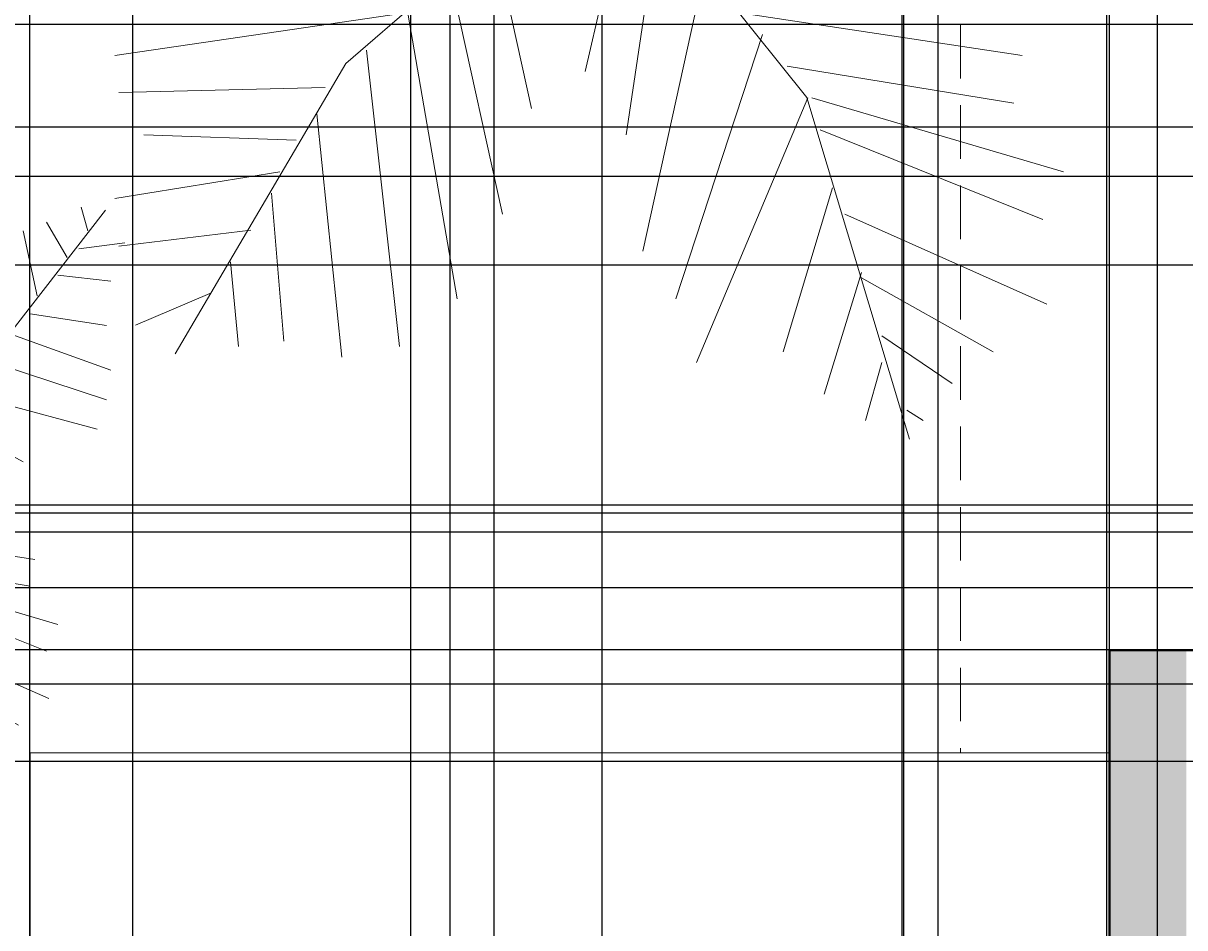
# Model space of a CAD drawing. Units: inches. Extents: x 818 to 1898, y 976 to 2364.
# Tile 11 of 96: x 1071 to 1207, y 1668 to 1773. Entities that reach past the tile are written whole.
import ezdxf

# ---------------------------------------------------------------- set-up
doc = ezdxf.new("R2010")
doc.units = ezdxf.units.IN
doc.header["$LTSCALE"] = 5
doc.header["$MEASUREMENT"] = 0
doc.linetypes.add('HIDDEN', pattern=[0.375, 0.25, -0.125])
for name, color, linetype, lineweight in [('A-ANNO-DIMS', 2, 'Continuous', 18), ('A-FLOR-OVHD', 8, 'HIDDEN', 13), ('A-WALL', 7, 'Continuous', 40), ('L-PAVE', 8, 'Continuous', 18), ('L-PLNT-BEDS', 94, 'Continuous', 18)]:
    doc.layers.add(name, color=color, linetype=linetype, lineweight=lineweight)
doc.layers.add('A-WALL-PATT', color=251, linetype='Continuous', lineweight=13, true_color=0x636466)
doc.layers.add('L-PLNT', color=116, linetype='Continuous', lineweight=13, true_color=0x136734)
doc.styles.get("Standard").update_dxf_attribs({"font": 'arial.ttf'})
doc.dimstyles.get("Standard").update_dxf_attribs({"dimtxt": 0.18, "dimasz": 0.18, "dimexe": 0.18, "dimexo": 0.0625, "dimgap": 0.09, "dimtad": 0, "dimtih": 1, "dimtoh": 1, "dimdec": 4, "dimzin": 0, "dimdsep": 46, "dimtxsty": 'Standard', "dimcen": 0.09, "dimadec": 0, "dimazin": 0, "dimtfac": 1, "dimtdec": 4, "dimtofl": 0, "dimtmove": 0, "dimatfit": 3, "dimfxl": 1, "dimtolj": 1, "dimtzin": 0, "dimarcsym": 0})

# ---------------------------------------------------------------- blocks, each defined once
blk = doc.blocks.new('PALM-BORDER')
for p, q in [((41.53, 39.05), (33.72, 81.45)), ((33.95, 78.95), (31.8, 80.68)), ((34.76, 77.57), (36.65, 80.68)), ((35.03, 74.11), (28.83, 78.26)), ((35.84, 71.35), (39.61, 75.84)), ((37.18, 65.82), (45, 74.8)), ((36.11, 68.59), (25.33, 73.77)), ((37.72, 59.6), (49.31, 73.77)), ((37.72, 59.95), (23.17, 69.28)), ((39.34, 51.31), (47.96, 67.2)), ((38.8, 53.39), (21.02, 65.48)), ((61.61, 45.75), (77.23, 65.83)), ((61.71, 45.79), (64.67, 65.82)), ((74.37, 66.17), (75.18, 63.4)), ((70.33, 64.44), (72.75, 60.3)), ((53.62, 43.37), (58.74, 62.37)), ((57.93, 44.41), (61.97, 63.06)), ((67.63, 63.4), (69.25, 55.81)), ((65.21, 62.02), (65.75, 51.31)), ((74.1, 61.33), (79.49, 62.02)), ((5.39, 54.77), (4.85, 60.64)), ((9.16, 60.3), (9.97, 50.62)), ((15.09, 59.95), (23.44, 41.99)), ((12.93, 58.57), (15.63, 44.75)), ((40.69, 44.06), (48.23, 58.91)), ((49.04, 41.64), (54.7, 58.57)), ((18.1, 42.4), (2.48, 58.02)), ((30.72, 40.61), (18.59, 57.88)), ((44.46, 40.26), (49.85, 57.19)), ((71.68, 58.22), (77.87, 57.53)), ((23.44, 56.84), (39.34, 49.24)), ((6.2, 53.73), (0, 52.7)), ((68.44, 53.73), (77.33, 52.35)), ((66.29, 51.31), (77.87, 47.17)), ((11.32, 49.24), (0.54, 47.17)), ((26.14, 49.24), (40.69, 42.68)), ((63.59, 48.21), (77.33, 43.71)), ((41.53, 39.05), (61.61, 45.75)), ((59.55, 44.75), (76.26, 40.26)), ((16.71, 43.71), (2.69, 43.02)), ((41.53, 39.05), (18.1, 42.4)), ((54.97, 43.37), (67.63, 36.46)), ((20.48, 41.64), (5.93, 34.73)), ((25.6, 41.3), (13.2, 33.01)), ((49.85, 41.64), (64.4, 34.73)), ((29.64, 40.61), (19.13, 31.97)), ((36.65, 39.91), (25.6, 33.01)), ((46.35, 40.26), (60.9, 32.66)), ((41.53, 39.05), (24.79, 24.55)), ((41.53, 39.05), (54.92, 22.32)), ((43.38, 36.81), (40.42, 24.02)), ((42.84, 37.15), (59.55, 31.97)), ((37.99, 36.46), (38.8, 28.17)), ((36.65, 34.73), (26.68, 31.62)), ((45.27, 34.39), (43.11, 19.88)), ((34.49, 32.66), (36.92, 21.61)), ((47.15, 32.32), (65.48, 28.17)), ((31.53, 30.59), (35.03, 14.7)), ((48.23, 30.59), (44.19, 12.28)), ((30.18, 29.55), (19.13, 29.55)), ((28.56, 27.82), (9.7, 25.06)), ((28.83, 27.82), (32.07, 9.17)), ((50.66, 27.82), (68.98, 25.06)), ((52, 26.44), (46.35, 9.17)), ((24.79, 24.55), (13.63, 5.58)), ((26.14, 25.41), (28.29, 6.06)), ((53.62, 24.37), (68.44, 21.95)), ((23.44, 22.99), (9.97, 22.64)), ((54.97, 22.3), (47.69, 5.02)), ((54.92, 22.32), (61.61, 0)), ((55.24, 22.3), (71.68, 17.46)), ((22.9, 21.26), (24.52, 5.37)), ((21.56, 19.53), (11.59, 19.88)), ((55.78, 20.22), (70.33, 14.35)), ((20.48, 17.46), (9.7, 15.73)), ((56.59, 16.42), (53.35, 5.72)), ((19.94, 16.08), (20.75, 6.41)), ((18.59, 13.66), (9.97, 12.62)), ((57.39, 14.7), (70.6, 8.83)), ((17.24, 11.59), (17.78, 6.06)), ((58.47, 10.9), (56.05, 2.95)), ((15.9, 9.52), (11.05, 7.44)), ((58.47, 10.55), (67.09, 5.72)), ((59.82, 6.75), (64.4, 3.64)), ((59.82, 5.02), (58.74, 1.22)), ((61.44, 1.92), (62.51, 1.22))]:
    blk.add_line(p, q)
blk = doc.blocks.new('PALM-DECK')
for p, q in [((74.19, 69.77), (44.29, 43.85)), ((74.19, 69.77), (98.11, 39.87)), ((77.51, 65.76), (72.21, 42.92)), ((80.88, 61.44), (77.03, 35.52)), ((61.62, 58.35), (65.95, 38.6)), ((56.33, 54.65), (62.58, 26.26)), ((86.17, 54.65), (78.95, 21.94)), ((51.03, 49.71), (17.33, 44.77)), ((51.51, 49.71), (57.29, 16.38)), ((90.51, 49.71), (123.24, 44.77)), ((92.91, 47.24), (82.8, 16.38)), ((46.7, 45.39), (50.55, 10.83)), ((44.29, 43.85), (24.36, 9.97)), ((95.8, 43.54), (122.28, 39.22)), ((41.88, 41.07), (17.81, 40.45)), ((98.21, 39.84), (85.21, 8.98)), ((98.11, 39.87), (110.08, 0)), ((98.69, 39.84), (128.06, 31.2)), ((40.92, 37.98), (43.81, 9.59)), ((38.51, 34.9), (20.7, 35.52)), ((99.65, 36.13), (125.65, 25.64)), ((36.59, 31.2), (17.33, 28.11)), ((35.62, 28.73), (37.07, 11.45)), ((101.1, 29.34), (95.32, 10.21)), ((102.54, 26.26), (126.13, 15.77)), ((33.22, 24.41), (17.81, 22.55)), ((30.81, 20.7), (31.77, 10.83)), ((104.47, 19.47), (100.13, 5.27)), ((104.47, 18.85), (119.87, 10.21)), ((28.4, 17), (19.74, 13.3)), ((106.87, 12.06), (115.06, 6.51)), ((106.87, 8.98), (104.95, 2.19)), ((109.76, 3.42), (111.69, 2.19))]:
    blk.add_line(p, q)
blk = doc.blocks.new('*D59')
at = {"layer": 'A-ANNO-DIMS', "color": 0, "lineweight": -2, "ltscale": 5, "transparency": 16777216}
for p, q in [((1251.64, 2300.39), (818.03, 2300.39)), ((818.21, 2300.21), (818.21, 1669.95)), ((818.21, 1039.32), (818.21, 1669.59)), ((896.05, 1039.14), (818.03, 1039.14))]:
    blk.add_line(p, q, dxfattribs=at)
at = {"layer": 'A-ANNO-DIMS', "color": 0, "ltscale": 5, "transparency": 16777216}
for points in [[(818.18, 2300.21), (818.24, 2300.21), (818.21, 2300.39)], [(818.18, 1039.32), (818.24, 1039.32), (818.21, 1039.14)]]:
    blk.add_solid(points, dxfattribs=at)
at = {"layer": 'Defpoints', "color": 0, "ltscale": 5, "transparency": 16777216}
for p in [(818.21, 2300.39), (1251.71, 2300.39), (896.11, 1039.14)]:
    blk.add_point(p, dxfattribs=at)
at = {"layer": 'A-ANNO-DIMS', "color": 0, "ltscale": 5, "transparency": 16777216, "insert": (818.21, 1669.77), "char_height": 0.18, "attachment_point": 5}
blk.add_mtext('\\A1;1261.2', dxfattribs=at)
blk = doc.blocks.new('*D61')
at = {"layer": 'A-ANNO-DIMS', "color": 0, "lineweight": -2, "ltscale": 5, "transparency": 16777216}
for p, q in [((1071.73, 1203.03), (1071.73, 2363.87)), ((1071.91, 2363.69), (1250.94, 2363.69)), ((1430.55, 2363.69), (1251.51, 2363.69)), ((1430.73, 1203.03), (1430.73, 2363.87))]:
    blk.add_line(p, q, dxfattribs=at)
at = {"layer": 'A-ANNO-DIMS', "color": 0, "ltscale": 5, "transparency": 16777216}
for points in [[(1071.91, 2363.72), (1071.91, 2363.66), (1071.73, 2363.69)], [(1430.55, 2363.72), (1430.55, 2363.66), (1430.73, 2363.69)]]:
    blk.add_solid(points, dxfattribs=at)
at = {"layer": 'Defpoints', "color": 0, "ltscale": 5, "transparency": 16777216}
for p in [(1430.73, 2363.69), (1071.73, 1202.96), (1430.73, 1202.96)]:
    blk.add_point(p, dxfattribs=at)
at = {"layer": 'A-ANNO-DIMS', "color": 0, "ltscale": 5, "transparency": 16777216, "insert": (1251.23, 2363.69), "char_height": 0.18, "attachment_point": 5}
blk.add_mtext('\\A1;359', dxfattribs=at)
blk = doc.blocks.new('*D64')
at = {"layer": 'A-ANNO-DIMS', "color": 0, "lineweight": -2, "ltscale": 5, "transparency": 16777216}
for p, q in [((1197.73, 1501.14), (1197.73, 2363.87)), ((1197.91, 2363.69), (1313.93, 2363.69)), ((1430.55, 2363.69), (1314.52, 2363.69)), ((1430.73, 1501.14), (1430.73, 2363.87))]:
    blk.add_line(p, q, dxfattribs=at)
at = {"layer": 'A-ANNO-DIMS', "color": 0, "ltscale": 5, "transparency": 16777216}
for points in [[(1197.91, 2363.72), (1197.91, 2363.66), (1197.73, 2363.69)], [(1430.55, 2363.72), (1430.55, 2363.66), (1430.73, 2363.69)]]:
    blk.add_solid(points, dxfattribs=at)
at = {"layer": 'Defpoints', "color": 0, "ltscale": 5, "transparency": 16777216}
for p in [(1430.73, 2363.69), (1197.73, 1501.08), (1430.73, 1501.08)]:
    blk.add_point(p, dxfattribs=at)
at = {"layer": 'A-ANNO-DIMS', "color": 0, "ltscale": 5, "transparency": 16777216, "insert": (1314.23, 2363.69), "char_height": 0.18, "attachment_point": 5}
blk.add_mtext('\\A1;233', dxfattribs=at)
blk = doc.blocks.new('*D79')
at = {"layer": 'A-ANNO-DIMS', "color": 0, "lineweight": -2, "ltscale": 5, "transparency": 16777216}
for p, q in [((992.73, 1203.03), (992.73, 2363.87)), ((992.91, 2363.69), (1032.01, 2363.69)), ((1071.55, 2363.69), (1032.44, 2363.69)), ((1071.73, 1203.03), (1071.73, 2363.87))]:
    blk.add_line(p, q, dxfattribs=at)
at = {"layer": 'A-ANNO-DIMS', "color": 0, "ltscale": 5, "transparency": 16777216}
for points in [[(992.91, 2363.72), (992.91, 2363.66), (992.73, 2363.69)], [(1071.55, 2363.72), (1071.55, 2363.66), (1071.73, 2363.69)]]:
    blk.add_solid(points, dxfattribs=at)
at = {"layer": 'Defpoints', "color": 0, "ltscale": 5, "transparency": 16777216}
for p in [(1071.73, 2363.69), (992.73, 1202.96), (1071.73, 1202.96)]:
    blk.add_point(p, dxfattribs=at)
at = {"layer": 'A-ANNO-DIMS', "color": 0, "ltscale": 5, "transparency": 16777216, "insert": (1032.23, 2363.69), "char_height": 0.18, "attachment_point": 5}
blk.add_mtext('\\A1;79', dxfattribs=at)
blk = doc.blocks.new('*D82')
at = {"layer": 'A-ANNO-DIMS', "color": 0, "lineweight": -2, "ltscale": 5, "transparency": 16777216}
for p, q in [((1083.73, 1501.14), (1083.73, 2363.87)), ((1083.91, 2363.69), (1140.45, 2363.69)), ((1197.55, 2363.69), (1141.01, 2363.69)), ((1197.73, 1501.14), (1197.73, 2363.87))]:
    blk.add_line(p, q, dxfattribs=at)
at = {"layer": 'A-ANNO-DIMS', "color": 0, "ltscale": 5, "transparency": 16777216}
for points in [[(1083.91, 2363.72), (1083.91, 2363.66), (1083.73, 2363.69)], [(1197.55, 2363.72), (1197.55, 2363.66), (1197.73, 2363.69)]]:
    blk.add_solid(points, dxfattribs=at)
at = {"layer": 'Defpoints', "color": 0, "ltscale": 5, "transparency": 16777216}
for p in [(1197.73, 2363.69), (1083.73, 1501.08), (1197.73, 1501.08)]:
    blk.add_point(p, dxfattribs=at)
at = {"layer": 'A-ANNO-DIMS', "color": 0, "ltscale": 5, "transparency": 16777216, "insert": (1140.73, 2363.69), "char_height": 0.18, "attachment_point": 5}
blk.add_mtext('\\A1;114', dxfattribs=at)
blk = doc.blocks.new('*D83')
at = {"layer": 'A-ANNO-DIMS', "color": 0, "lineweight": -2, "ltscale": 5, "transparency": 16777216}
for p, q in [((1197.73, 1700.14), (1197.73, 2363.87)), ((1197.91, 2363.69), (1228.02, 2363.69)), ((1258.55, 2363.69), (1228.43, 2363.69)), ((1258.73, 1700.14), (1258.73, 2363.87))]:
    blk.add_line(p, q, dxfattribs=at)
at = {"layer": 'A-ANNO-DIMS', "color": 0, "ltscale": 5, "transparency": 16777216}
for points in [[(1197.91, 2363.72), (1197.91, 2363.66), (1197.73, 2363.69)], [(1258.55, 2363.72), (1258.55, 2363.66), (1258.73, 2363.69)]]:
    blk.add_solid(points, dxfattribs=at)
at = {"layer": 'Defpoints', "color": 0, "ltscale": 5, "transparency": 16777216}
for p in [(1258.73, 2363.69), (1197.73, 1700.08), (1258.73, 1700.08)]:
    blk.add_point(p, dxfattribs=at)
at = {"layer": 'A-ANNO-DIMS', "color": 0, "ltscale": 5, "transparency": 16777216, "insert": (1228.23, 2363.69), "char_height": 0.18, "attachment_point": 5}
blk.add_mtext('\\A1;61', dxfattribs=at)
blk = doc.blocks.new('*D84')
at = {"layer": 'A-ANNO-DIMS', "color": 0, "lineweight": -2, "ltscale": 5, "transparency": 16777216}
for p, q in [((1197.66, 1700.08), (818.03, 1700.08)), ((818.21, 1699.9), (818.21, 1600.76)), ((818.21, 1501.26), (818.21, 1600.4)), ((1197.66, 1501.08), (818.03, 1501.08))]:
    blk.add_line(p, q, dxfattribs=at)
at = {"layer": 'A-ANNO-DIMS', "color": 0, "ltscale": 5, "transparency": 16777216}
for points in [[(818.18, 1699.9), (818.24, 1699.9), (818.21, 1700.08)], [(818.18, 1501.26), (818.24, 1501.26), (818.21, 1501.08)]]:
    blk.add_solid(points, dxfattribs=at)
at = {"layer": 'Defpoints', "color": 0, "ltscale": 5, "transparency": 16777216}
for p in [(818.21, 1700.08), (1197.73, 1700.08), (1197.73, 1501.08)]:
    blk.add_point(p, dxfattribs=at)
at = {"layer": 'A-ANNO-DIMS', "color": 0, "ltscale": 5, "transparency": 16777216, "insert": (818.21, 1600.58), "char_height": 0.18, "attachment_point": 5}
blk.add_mtext('\\A1;199', dxfattribs=at)
blk = doc.blocks.new('*D93')
at = {"layer": 'A-ANNO-DIMS', "color": 0, "lineweight": -2, "ltscale": 5, "transparency": 16777216}
for p, q in [((1068.34, 1071.12), (1068.34, 2363.87)), ((1068.52, 2363.69), (1094.16, 2363.69)), ((1120.58, 2363.69), (1094.94, 2363.69)), ((1120.76, 1071.12), (1120.76, 2363.87))]:
    blk.add_line(p, q, dxfattribs=at)
at = {"layer": 'A-ANNO-DIMS', "color": 0, "ltscale": 5, "transparency": 16777216}
for points in [[(1068.52, 2363.72), (1068.52, 2363.66), (1068.34, 2363.69)], [(1120.58, 2363.72), (1120.58, 2363.66), (1120.76, 2363.69)]]:
    blk.add_solid(points, dxfattribs=at)
at = {"layer": 'Defpoints', "color": 0, "ltscale": 5, "transparency": 16777216}
for p in [(1120.76, 2363.69), (1068.34, 1071.06), (1120.76, 1071.06)]:
    blk.add_point(p, dxfattribs=at)
at = {"layer": 'A-ANNO-DIMS', "color": 0, "ltscale": 5, "transparency": 16777216, "insert": (1094.55, 2363.69), "char_height": 0.18, "attachment_point": 5}
blk.add_mtext('\\A1;52.42', dxfattribs=at)
blk = doc.blocks.new('*D94')
at = {"layer": 'A-ANNO-DIMS', "color": 0, "lineweight": -2, "ltscale": 5, "transparency": 16777216}
for p, q in [((1120.76, 1071.12), (1120.76, 2363.87)), ((1120.94, 2363.69), (1146.76, 2363.69)), ((1173.36, 2363.69), (1147.55, 2363.69)), ((1173.54, 1071.12), (1173.54, 2363.87))]:
    blk.add_line(p, q, dxfattribs=at)
at = {"layer": 'A-ANNO-DIMS', "color": 0, "ltscale": 5, "transparency": 16777216}
for points in [[(1120.94, 2363.72), (1120.94, 2363.66), (1120.76, 2363.69)], [(1173.36, 2363.72), (1173.36, 2363.66), (1173.54, 2363.69)]]:
    blk.add_solid(points, dxfattribs=at)
at = {"layer": 'Defpoints', "color": 0, "ltscale": 5, "transparency": 16777216}
for p in [(1173.54, 2363.69), (1120.76, 1071.06), (1173.54, 1071.06)]:
    blk.add_point(p, dxfattribs=at)
at = {"layer": 'A-ANNO-DIMS', "color": 0, "ltscale": 5, "transparency": 16777216, "insert": (1147.15, 2363.69), "char_height": 0.18, "attachment_point": 5}
blk.add_mtext('\\A1;52.78', dxfattribs=at)
blk = doc.blocks.new('*D95')
at = {"layer": 'A-ANNO-DIMS', "color": 0, "lineweight": -2, "ltscale": 5, "transparency": 16777216}
for p, q in [((1173.54, 1071.12), (1173.54, 2363.87)), ((1173.72, 2363.69), (1201.29, 2363.69)), ((1229.47, 2363.69), (1201.9, 2363.69)), ((1229.65, 1071.12), (1229.65, 2363.87))]:
    blk.add_line(p, q, dxfattribs=at)
at = {"layer": 'A-ANNO-DIMS', "color": 0, "ltscale": 5, "transparency": 16777216}
for points in [[(1173.72, 2363.72), (1173.72, 2363.66), (1173.54, 2363.69)], [(1229.47, 2363.72), (1229.47, 2363.66), (1229.65, 2363.69)]]:
    blk.add_solid(points, dxfattribs=at)
at = {"layer": 'Defpoints', "color": 0, "ltscale": 5, "transparency": 16777216}
for p in [(1229.65, 2363.69), (1173.54, 1071.06), (1229.65, 1071.06)]:
    blk.add_point(p, dxfattribs=at)
at = {"layer": 'A-ANNO-DIMS', "color": 0, "ltscale": 5, "transparency": 16777216, "insert": (1201.59, 2363.69), "char_height": 0.18, "attachment_point": 5}
blk.add_mtext('\\A1;56.1', dxfattribs=at)
blk = doc.blocks.new('*D109')
at = {"layer": 'A-ANNO-DIMS', "color": 0, "lineweight": -2, "ltscale": 5, "transparency": 16777216}
for p, q in [((1125.92, 1410.12), (1125.92, 2363.87)), ((1126.1, 2363.69), (1164.25, 2363.69)), ((1203.15, 2363.69), (1165, 2363.69)), ((1203.33, 1409.91), (1203.33, 2363.87))]:
    blk.add_line(p, q, dxfattribs=at)
at = {"layer": 'A-ANNO-DIMS', "color": 0, "ltscale": 5, "transparency": 16777216}
for points in [[(1126.1, 2363.72), (1126.1, 2363.66), (1125.92, 2363.69)], [(1203.15, 2363.72), (1203.15, 2363.66), (1203.33, 2363.69)]]:
    blk.add_solid(points, dxfattribs=at)
at = {"layer": 'Defpoints', "color": 0, "ltscale": 5, "transparency": 16777216}
for p in [(1203.33, 2363.69), (1125.92, 1410.05), (1203.33, 1409.85)]:
    blk.add_point(p, dxfattribs=at)
at = {"layer": 'A-ANNO-DIMS', "color": 0, "ltscale": 5, "transparency": 16777216, "insert": (1164.62, 2363.69), "char_height": 0.18, "attachment_point": 5}
blk.add_mtext('\\A1;77.41', dxfattribs=at)
blk = doc.blocks.new('*D119')
at = {"layer": 'A-ANNO-DIMS', "color": 0, "lineweight": -2, "ltscale": 5, "transparency": 16777216}
for p, q in [((1766.29, 1716.99), (818.03, 1716.99)), ((818.21, 1716.81), (818.21, 1672.43)), ((818.21, 1627.69), (818.21, 1672.06)), ((1766.29, 1627.51), (818.03, 1627.51))]:
    blk.add_line(p, q, dxfattribs=at)
at = {"layer": 'A-ANNO-DIMS', "color": 0, "ltscale": 5, "transparency": 16777216}
for points in [[(818.18, 1716.81), (818.24, 1716.81), (818.21, 1716.99)], [(818.18, 1627.69), (818.24, 1627.69), (818.21, 1627.51)]]:
    blk.add_solid(points, dxfattribs=at)
at = {"layer": 'Defpoints', "color": 0, "ltscale": 5, "transparency": 16777216}
for p in [(818.21, 1716.99), (1766.35, 1716.99), (1766.35, 1627.51)]:
    blk.add_point(p, dxfattribs=at)
at = {"layer": 'A-ANNO-DIMS', "color": 0, "ltscale": 5, "transparency": 16777216, "insert": (818.21, 1672.25), "char_height": 0.18, "attachment_point": 5}
blk.add_mtext('\\A1;89.48', dxfattribs=at)
blk = doc.blocks.new('*D120')
at = {"layer": 'A-ANNO-DIMS', "color": 0, "lineweight": -2, "ltscale": 5, "transparency": 16777216}
for p, q in [((1766.29, 1797.72), (818.03, 1797.72)), ((818.21, 1797.54), (818.21, 1757.53)), ((818.21, 1717.17), (818.21, 1757.17)), ((1766.29, 1716.99), (818.03, 1716.99))]:
    blk.add_line(p, q, dxfattribs=at)
at = {"layer": 'A-ANNO-DIMS', "color": 0, "ltscale": 5, "transparency": 16777216}
for points in [[(818.18, 1797.54), (818.24, 1797.54), (818.21, 1797.72)], [(818.18, 1717.17), (818.24, 1717.17), (818.21, 1716.99)]]:
    blk.add_solid(points, dxfattribs=at)
at = {"layer": 'Defpoints', "color": 0, "ltscale": 5, "transparency": 16777216}
for p in [(818.21, 1797.72), (1766.35, 1797.72), (1766.35, 1716.99)]:
    blk.add_point(p, dxfattribs=at)
at = {"layer": 'A-ANNO-DIMS', "color": 0, "ltscale": 5, "transparency": 16777216, "insert": (818.21, 1757.35), "char_height": 0.18, "attachment_point": 5}
blk.add_mtext('\\A1;80.73', dxfattribs=at)
blk = doc.blocks.new('*D122')
at = {"layer": 'A-ANNO-DIMS', "color": 0, "lineweight": -2, "ltscale": 5, "transparency": 16777216}
for p, q in [((1138.5, 1794.37), (1138.5, 975.66)), ((1071.73, 1688.02), (1071.73, 975.66)), ((1071.91, 975.84), (1104.72, 975.84)), ((1138.32, 975.84), (1105.51, 975.84))]:
    blk.add_line(p, q, dxfattribs=at)
at = {"layer": 'A-ANNO-DIMS', "color": 0, "ltscale": 5, "transparency": 16777216}
for points in [[(1071.91, 975.87), (1071.91, 975.81), (1071.73, 975.84)], [(1138.32, 975.87), (1138.32, 975.81), (1138.5, 975.84)]]:
    blk.add_solid(points, dxfattribs=at)
at = {"layer": 'Defpoints', "color": 0, "ltscale": 5, "transparency": 16777216}
for p in [(1138.5, 1794.43), (1071.73, 1688.08), (1138.5, 975.84)]:
    blk.add_point(p, dxfattribs=at)
at = {"layer": 'A-ANNO-DIMS', "color": 0, "ltscale": 5, "transparency": 16777216, "insert": (1105.11, 975.84), "char_height": 0.18, "attachment_point": 5}
blk.add_mtext('\\A1;66.78', dxfattribs=at)
blk = doc.blocks.new('*D126')
at = {"layer": 'A-ANNO-DIMS', "color": 0, "lineweight": -2, "ltscale": 5, "transparency": 16777216}
for p, q in [((1035.38, 1252.09), (1035.38, 2363.87)), ((1035.56, 2363.69), (1075.41, 2363.69)), ((1116.01, 2363.69), (1076.16, 2363.69)), ((1116.19, 1236.03), (1116.19, 2363.87))]:
    blk.add_line(p, q, dxfattribs=at)
at = {"layer": 'A-ANNO-DIMS', "color": 0, "ltscale": 5, "transparency": 16777216}
for points in [[(1035.56, 2363.72), (1035.56, 2363.66), (1035.38, 2363.69)], [(1116.01, 2363.72), (1116.01, 2363.66), (1116.19, 2363.69)]]:
    blk.add_solid(points, dxfattribs=at)
at = {"layer": 'Defpoints', "color": 0, "ltscale": 5, "transparency": 16777216}
for p in [(1035.38, 2363.69), (1035.38, 1252.02), (1116.19, 1235.96)]:
    blk.add_point(p, dxfattribs=at)
at = {"layer": 'A-ANNO-DIMS', "color": 0, "ltscale": 5, "transparency": 16777216, "insert": (1075.78, 2363.69), "char_height": 0.18, "attachment_point": 5}
blk.add_mtext('\\A1;80.81', dxfattribs=at)
blk = doc.blocks.new('*D145')
at = {"layer": 'A-ANNO-DIMS', "color": 0, "lineweight": -2, "ltscale": 5, "transparency": 16777216}
for p, q in [((1197.39, 2122.31), (1197.39, 975.66)), ((1232.61, 2122.31), (1232.61, 975.66)), ((1197.57, 975.84), (1214.61, 975.84)), ((1232.43, 975.84), (1215.39, 975.84))]:
    blk.add_line(p, q, dxfattribs=at)
at = {"layer": 'A-ANNO-DIMS', "color": 0, "ltscale": 5, "transparency": 16777216}
for points in [[(1197.57, 975.87), (1197.57, 975.81), (1197.39, 975.84)], [(1232.43, 975.87), (1232.43, 975.81), (1232.61, 975.84)]]:
    blk.add_solid(points, dxfattribs=at)
at = {"layer": 'Defpoints', "color": 0, "ltscale": 5, "transparency": 16777216}
for p in [(1197.39, 2122.38), (1232.61, 2122.38), (1232.61, 975.84)]:
    blk.add_point(p, dxfattribs=at)
at = {"layer": 'A-ANNO-DIMS', "color": 0, "ltscale": 5, "transparency": 16777216, "insert": (1215, 975.84), "char_height": 0.18, "attachment_point": 5}
blk.add_mtext('\\A1;35.22', dxfattribs=at)
blk = doc.blocks.new('*D158')
at = {"layer": 'A-ANNO-DIMS', "color": 0, "lineweight": -2, "ltscale": 5, "transparency": 16777216}
for p, q in [((1173.73, 1590.82), (1173.73, 2363.87)), ((1173.91, 2363.69), (1175.57, 2363.69)), ((1177.55, 2363.69), (1175.88, 2363.69)), ((1177.73, 1586.82), (1177.73, 2363.87))]:
    blk.add_line(p, q, dxfattribs=at)
at = {"layer": 'A-ANNO-DIMS', "color": 0, "ltscale": 5, "transparency": 16777216}
for points in [[(1173.91, 2363.72), (1173.91, 2363.66), (1173.73, 2363.69)], [(1177.55, 2363.72), (1177.55, 2363.66), (1177.73, 2363.69)]]:
    blk.add_solid(points, dxfattribs=at)
at = {"layer": 'Defpoints', "color": 0, "ltscale": 5, "transparency": 16777216}
for p in [(1177.73, 2363.69), (1173.73, 1590.76), (1177.73, 1586.76)]:
    blk.add_point(p, dxfattribs=at)
at = {"layer": 'A-ANNO-DIMS', "color": 0, "ltscale": 5, "transparency": 16777216, "insert": (1175.73, 2363.69), "char_height": 0.18, "attachment_point": 5}
blk.add_mtext('\\A1;4', dxfattribs=at)
blk = doc.blocks.new('*D176')
at = {"layer": 'A-ANNO-DIMS', "color": 0, "lineweight": -2, "ltscale": 5, "transparency": 16777216}
for p, q in [((1559.66, 1687.08), (818.03, 1687.08)), ((818.21, 1686.9), (818.21, 1667.51)), ((818.21, 1647.76), (818.21, 1667.15)), ((1559.66, 1647.58), (818.03, 1647.58))]:
    blk.add_line(p, q, dxfattribs=at)
at = {"layer": 'A-ANNO-DIMS', "color": 0, "ltscale": 5, "transparency": 16777216}
for points in [[(818.18, 1686.9), (818.24, 1686.9), (818.21, 1687.08)], [(818.18, 1647.76), (818.24, 1647.76), (818.21, 1647.58)]]:
    blk.add_solid(points, dxfattribs=at)
at = {"layer": 'Defpoints', "color": 0, "ltscale": 5, "transparency": 16777216}
for p in [(1559.73, 1687.08), (818.21, 1647.58), (1559.73, 1647.58)]:
    blk.add_point(p, dxfattribs=at)
at = {"layer": 'A-ANNO-DIMS', "color": 0, "ltscale": 5, "transparency": 16777216, "insert": (818.21, 1667.33), "char_height": 0.18, "attachment_point": 5}
blk.add_mtext('\\A1;39.5', dxfattribs=at)
blk = doc.blocks.new('*D215')
at = {"layer": 'A-ANNO-DIMS', "color": 0, "lineweight": -2, "ltscale": 5, "transparency": 16777216}
for p, q in [((1590.66, 1876.08), (818.03, 1876.08)), ((818.21, 1875.9), (818.21, 1781.76)), ((818.21, 1687.26), (818.21, 1781.4)), ((1511.66, 1687.08), (818.03, 1687.08))]:
    blk.add_line(p, q, dxfattribs=at)
at = {"layer": 'A-ANNO-DIMS', "color": 0, "ltscale": 5, "transparency": 16777216}
for points in [[(818.18, 1875.9), (818.24, 1875.9), (818.21, 1876.08)], [(818.18, 1687.26), (818.24, 1687.26), (818.21, 1687.08)]]:
    blk.add_solid(points, dxfattribs=at)
at = {"layer": 'Defpoints', "color": 0, "ltscale": 5, "transparency": 16777216}
for p in [(818.21, 1876.08), (1590.73, 1876.08), (1511.73, 1687.08)]:
    blk.add_point(p, dxfattribs=at)
at = {"layer": 'A-ANNO-DIMS', "color": 0, "ltscale": 5, "transparency": 16777216, "insert": (818.21, 1781.58), "char_height": 0.18, "attachment_point": 5}
blk.add_mtext('\\A1;189', dxfattribs=at)
blk = doc.blocks.new('*D220')
at = {"layer": 'A-ANNO-DIMS', "color": 0, "lineweight": -2, "ltscale": 5, "transparency": 16777216}
for p, q in [((1520.66, 1773.08), (818.03, 1773.08)), ((818.21, 1772.9), (818.21, 1767.26)), ((818.21, 1761.26), (818.21, 1766.9)), ((1520.66, 1761.08), (818.03, 1761.08))]:
    blk.add_line(p, q, dxfattribs=at)
at = {"layer": 'A-ANNO-DIMS', "color": 0, "ltscale": 5, "transparency": 16777216}
for points in [[(818.18, 1772.9), (818.24, 1772.9), (818.21, 1773.08)], [(818.18, 1761.26), (818.24, 1761.26), (818.21, 1761.08)]]:
    blk.add_solid(points, dxfattribs=at)
at = {"layer": 'Defpoints', "color": 0, "ltscale": 5, "transparency": 16777216}
for p in [(818.21, 1773.08), (1520.73, 1773.08), (1520.73, 1761.08)]:
    blk.add_point(p, dxfattribs=at)
at = {"layer": 'A-ANNO-DIMS', "color": 0, "ltscale": 5, "transparency": 16777216, "insert": (818.21, 1767.08), "char_height": 0.18, "attachment_point": 5}
blk.add_mtext('\\A1;12', dxfattribs=at)
blk = doc.blocks.new('*D222')
at = {"layer": 'A-ANNO-DIMS', "color": 0, "lineweight": -2, "ltscale": 5, "transparency": 16777216}
for p, q in [((1511.66, 1744.97), (818.03, 1744.97)), ((818.21, 1744.79), (818.21, 1730.69)), ((818.21, 1716.23), (818.21, 1730.33)), ((1511.66, 1716.05), (818.03, 1716.05))]:
    blk.add_line(p, q, dxfattribs=at)
at = {"layer": 'A-ANNO-DIMS', "color": 0, "ltscale": 5, "transparency": 16777216}
for points in [[(818.18, 1744.79), (818.24, 1744.79), (818.21, 1744.97)], [(818.18, 1716.23), (818.24, 1716.23), (818.21, 1716.05)]]:
    blk.add_solid(points, dxfattribs=at)
at = {"layer": 'Defpoints', "color": 0, "ltscale": 5, "transparency": 16777216}
for p in [(818.21, 1744.97), (1511.73, 1744.97), (1511.73, 1716.05)]:
    blk.add_point(p, dxfattribs=at)
at = {"layer": 'A-ANNO-DIMS', "color": 0, "ltscale": 5, "transparency": 16777216, "insert": (818.21, 1730.51), "char_height": 0.18, "attachment_point": 5}
blk.add_mtext('\\A1;28.926', dxfattribs=at)
blk = doc.blocks.new('*D223')
at = {"layer": 'A-ANNO-DIMS', "color": 0, "lineweight": -2, "ltscale": 5, "transparency": 16777216}
for p, q in [((1511.66, 1716.05), (818.03, 1716.05)), ((818.21, 1715.87), (818.21, 1706.24)), ((818.21, 1696.26), (818.21, 1705.88)), ((1511.66, 1696.08), (818.03, 1696.08))]:
    blk.add_line(p, q, dxfattribs=at)
at = {"layer": 'A-ANNO-DIMS', "color": 0, "ltscale": 5, "transparency": 16777216}
for points in [[(818.18, 1715.87), (818.24, 1715.87), (818.21, 1716.05)], [(818.18, 1696.26), (818.24, 1696.26), (818.21, 1696.08)]]:
    blk.add_solid(points, dxfattribs=at)
at = {"layer": 'Defpoints', "color": 0, "ltscale": 5, "transparency": 16777216}
for p in [(818.21, 1716.05), (1511.73, 1716.05), (1511.73, 1696.08)]:
    blk.add_point(p, dxfattribs=at)
at = {"layer": 'A-ANNO-DIMS', "color": 0, "ltscale": 5, "transparency": 16777216, "insert": (818.21, 1706.06), "char_height": 0.18, "attachment_point": 5}
blk.add_mtext('\\A1;19.967', dxfattribs=at)
blk = doc.blocks.new('*D246')
at = {"layer": 'A-ANNO-DIMS', "color": 0, "lineweight": -2, "ltscale": 5, "transparency": 16777216}
for p, q in [((1258.66, 1755.33), (818.03, 1755.33)), ((818.21, 1755.15), (818.21, 1731.51)), ((818.21, 1707.51), (818.21, 1731.15)), ((1258.66, 1707.33), (818.03, 1707.33))]:
    blk.add_line(p, q, dxfattribs=at)
at = {"layer": 'A-ANNO-DIMS', "color": 0, "ltscale": 5, "transparency": 16777216}
for points in [[(818.18, 1755.15), (818.24, 1755.15), (818.21, 1755.33)], [(818.18, 1707.51), (818.24, 1707.51), (818.21, 1707.33)]]:
    blk.add_solid(points, dxfattribs=at)
at = {"layer": 'Defpoints', "color": 0, "ltscale": 5, "transparency": 16777216}
for p in [(818.21, 1755.33), (1258.73, 1755.33), (1258.73, 1707.33)]:
    blk.add_point(p, dxfattribs=at)
at = {"layer": 'A-ANNO-DIMS', "color": 0, "ltscale": 5, "transparency": 16777216, "insert": (818.21, 1731.33), "char_height": 0.18, "attachment_point": 5}
blk.add_mtext('\\A1;48', dxfattribs=at)
blk = doc.blocks.new('*D249')
at = {"layer": 'A-ANNO-DIMS', "color": 0, "lineweight": -2, "ltscale": 5, "transparency": 16777216}
for p, q in [((1258.66, 1814.97), (818.03, 1814.97)), ((818.21, 1814.79), (818.21, 1785.33)), ((818.21, 1755.51), (818.21, 1784.97)), ((1258.66, 1755.33), (818.03, 1755.33))]:
    blk.add_line(p, q, dxfattribs=at)
at = {"layer": 'A-ANNO-DIMS', "color": 0, "ltscale": 5, "transparency": 16777216}
for points in [[(818.18, 1814.79), (818.24, 1814.79), (818.21, 1814.97)], [(818.18, 1755.51), (818.24, 1755.51), (818.21, 1755.33)]]:
    blk.add_solid(points, dxfattribs=at)
at = {"layer": 'Defpoints', "color": 0, "ltscale": 5, "transparency": 16777216}
for p in [(818.21, 1814.97), (1258.73, 1814.97), (1258.73, 1755.33)]:
    blk.add_point(p, dxfattribs=at)
at = {"layer": 'A-ANNO-DIMS', "color": 0, "ltscale": 5, "transparency": 16777216, "insert": (818.21, 1785.15), "char_height": 0.18, "attachment_point": 5}
blk.add_mtext('\\A1;59.63', dxfattribs=at)
blk = doc.blocks.new('*D277')
at = {"layer": 'A-ANNO-DIMS', "color": 0, "lineweight": -2, "ltscale": 5, "transparency": 16777216}
for p, q in [((1251.87, 1687.08), (818.03, 1687.08)), ((818.21, 1686.9), (818.21, 1668.7)), ((818.21, 1650.13), (818.21, 1668.33)), ((1256.59, 1649.95), (818.03, 1649.95))]:
    blk.add_line(p, q, dxfattribs=at)
at = {"layer": 'A-ANNO-DIMS', "color": 0, "ltscale": 5, "transparency": 16777216}
for points in [[(818.18, 1686.9), (818.24, 1686.9), (818.21, 1687.08)], [(818.18, 1650.13), (818.24, 1650.13), (818.21, 1649.95)]]:
    blk.add_solid(points, dxfattribs=at)
at = {"layer": 'Defpoints', "color": 0, "ltscale": 5, "transparency": 16777216}
for p in [(818.21, 1687.08), (1251.93, 1687.08), (1256.65, 1649.95)]:
    blk.add_point(p, dxfattribs=at)
at = {"layer": 'A-ANNO-DIMS', "color": 0, "ltscale": 5, "transparency": 16777216, "insert": (818.21, 1668.52), "char_height": 0.18, "attachment_point": 5}
blk.add_mtext('\\A1;37.13', dxfattribs=at)
blk = doc.blocks.new('*D289')
at = {"layer": 'A-ANNO-DIMS', "color": 0, "lineweight": -2, "ltscale": 5, "transparency": 16777216}
for p, q in [((1279.06, 1713.82), (818.03, 1713.82)), ((818.21, 1713.64), (818.21, 1705.13)), ((818.21, 1696.26), (818.21, 1704.77)), ((1267.66, 1696.08), (818.03, 1696.08))]:
    blk.add_line(p, q, dxfattribs=at)
at = {"layer": 'A-ANNO-DIMS', "color": 0, "ltscale": 5, "transparency": 16777216}
for points in [[(818.18, 1713.64), (818.24, 1713.64), (818.21, 1713.82)], [(818.18, 1696.26), (818.24, 1696.26), (818.21, 1696.08)]]:
    blk.add_solid(points, dxfattribs=at)
at = {"layer": 'Defpoints', "color": 0, "ltscale": 5, "transparency": 16777216}
for p in [(1279.13, 1713.82), (818.21, 1696.08), (1267.73, 1696.08)]:
    blk.add_point(p, dxfattribs=at)
at = {"layer": 'A-ANNO-DIMS', "color": 0, "ltscale": 5, "transparency": 16777216, "insert": (818.21, 1704.95), "char_height": 0.18, "attachment_point": 5}
blk.add_mtext('\\A1;17.74', dxfattribs=at)

msp = doc.modelspace()

# ---------------------------------------------------------------- hatches: boundary and pattern name
at = {"layer": 'A-WALL-PATT', "ltscale": 5}
h = msp.add_hatch(color=256, dxfattribs=at)
h.dxf.hatch_style = 1
h.paths.add_polyline_path([(1206.7252, 1687.0782), (1206.7252, 1700.0782), (1197.7251, 1700.0782), (1197.7251, 1501.0782), (1206.7252, 1501.0782), (1206.7252, 1510.0782)])
h.paths.add_polyline_path([(1197.7251, 1590.7585), (1173.7251, 1590.7585), (1173.7251, 1586.7585), (1197.7251, 1586.7585)])
h.paths.add_polyline_path([(1197.7251, 1534.6024), (1173.7251, 1534.6024), (1173.7251, 1530.6024), (1197.7251, 1530.6024)])
h.paths.add_polyline_path([(1365.1463, 1510.0782), (1283.8183, 1510.0782), (1283.8183, 1501.0782), (1365.1463, 1501.0782)])
h.paths.add_polyline_path([(1439.7252, 1591.0782), (1441.7252, 1591.0782), (1441.7252, 1600.0782), (1430.7251, 1600.0782), (1430.7251, 1510.0782), (1406.7252, 1510.0782), (1401.1463, 1510.0782), (1401.1463, 1501.0782), (1430.7251, 1501.0782), (1430.7251, 1486.2383), (1430.7251, 1409.0522), (1439.7252, 1409.0522)])

# ---------------------------------------------------------------- linework, layer by layer
at = {"layer": 'A-FLOR-OVHD', "ltscale": 5}
msp.add_line((1180.349, 1913.6401), (1180.349, 1688.0782), dxfattribs=at)
at = {"layer": 'A-WALL'}
for q in [(1258.7251, 1700.0782), (1197.7251, 1501.0782)]:
    msp.add_line((1197.7251, 1700.0782), q, dxfattribs=at)
at = {"layer": 'L-PAVE'}
msp.add_line((1071.7251, 1688.0782), (1197.7251, 1688.0782), dxfattribs=at)
at = {"layer": 'L-PLNT-BEDS'}
for p, q in [((1071.7251, 2214.9709), (1071.7251, 1202.9642)), ((1083.7251, 2044.0782), (1083.7251, 1211.9642))]:
    msp.add_line(p, q, dxfattribs=at)

# ---------------------------------------------------------------- block references
at = {"layer": 'L-PLNT'}
for name, p in [('PALM-DECK', (1064.31, 1724.664)), ('PALM-BORDER', (1003.3185, 1685.5789))]:
    msp.add_blockref(name, p, dxfattribs=at)

# ---------------------------------------------------------------- dimensions: what is measured, and where the dimension line sits
at = {"layer": 'A-ANNO-DIMS', "ltscale": 5}
for base, p1, p2, override, picture, middle in [((1071.7251, 2363.6929), (992.7251, 1202.9642), (1071.7251, 1202.9642), {"dimdec": 0, "dimlfac": 1, "dimrnd": 0, "dimzin": 0, "dimdsep": 46, "dimlunit": 2}, '*D79', (1032.2251, 2363.6929)), ((1035.3768, 2363.6929), (1116.1882, 1235.9642), (1035.3768, 1252.0242), {"dimdec": 2, "dimlfac": 1, "dimrnd": 0, "dimzin": 0, "dimdsep": 46, "dimlunit": 2}, '*D126', (1075.7825, 2363.6929)), ((1120.7618, 2363.6929), (1068.3377, 1071.0552), (1120.7618, 1071.0552), {"dimdec": 2, "dimlfac": 1, "dimrnd": 0, "dimzin": 0, "dimdsep": 46, "dimlunit": 2}, '*D93', (1094.5497, 2363.6929)), ((1430.7251, 2363.6929), (1071.7251, 1202.9642), (1430.7251, 1202.9642), {"dimdec": 0, "dimlfac": 1, "dimrnd": 0, "dimzin": 0, "dimdsep": 46, "dimlunit": 2}, '*D61', (1251.2251, 2363.6929)), ((1197.7251, 2363.6929), (1083.7251, 1501.0782), (1197.7251, 1501.0782), {"dimdec": 0, "dimlfac": 1, "dimrnd": 0, "dimzin": 0, "dimdsep": 46, "dimlunit": 2}, '*D82', (1140.7251, 2363.6929)), ((1173.5418, 2363.6929), (1120.7618, 1071.0552), (1173.5418, 1071.0552), {"dimdec": 2, "dimlfac": 1, "dimrnd": 0, "dimzin": 0, "dimdsep": 46, "dimlunit": 2}, '*D94', (1147.1518, 2363.6929)), ((1203.3292, 2363.6929), (1125.9172, 1410.0547), (1203.3292, 1409.8484), {"dimdec": 2, "dimlfac": 1, "dimrnd": 0, "dimzin": 0, "dimdsep": 46, "dimlunit": 2}, '*D109', (1164.6232, 2363.6929)), ((1229.6474, 2363.6929), (1173.5418, 1071.0552), (1229.6474, 1071.0552), {"dimdec": 1, "dimlfac": 1, "dimrnd": 0, "dimzin": 0, "dimdsep": 46, "dimlunit": 2}, '*D95', (1201.5946, 2363.6929)), ((1177.7251, 2363.6929), (1173.7251, 1590.7585), (1177.7251, 1586.7585), {"dimdec": 0, "dimlfac": 1, "dimrnd": 0, "dimzin": 0, "dimdsep": 46, "dimlunit": 2}, '*D158', (1175.7251, 2363.6929)), ((1430.7251, 2363.6929), (1197.7251, 1501.0782), (1430.7251, 1501.0782), {"dimdec": 0, "dimlfac": 1, "dimrnd": 0, "dimzin": 0, "dimdsep": 46, "dimlunit": 2}, '*D64', (1314.2251, 2363.6929)), ((1258.7251, 2363.6929), (1197.7251, 1700.0782), (1258.7251, 1700.0782), {"dimdec": 0, "dimlfac": 1, "dimrnd": 0, "dimzin": 0, "dimdsep": 46, "dimlunit": 2}, '*D83', (1228.2251, 2363.6929)), ((1232.6091, 975.8433), (1197.3925, 2122.3767), (1232.6091, 2122.3767), {"dimdec": 2, "dimlfac": 1, "dimrnd": 0, "dimzin": 0, "dimdsep": 46, "dimlunit": 2}, '*D145', (1215.0008, 975.8433)), ((1138.5041, 975.8433), (1071.7251, 1688.0782), (1138.5041, 1794.4325), {"dimdec": 2, "dimlfac": 1, "dimrnd": 0, "dimzin": 0, "dimdsep": 46, "dimlunit": 2}, '*D122', (1105.1146, 975.8433))]:
    dim = msp.add_linear_dim(base=base, p1=p1, p2=p2, dimstyle='Standard', override=override, dxfattribs=at)
    dim.commit()
    dim.dimension.update_dxf_attribs({"geometry": picture, "text_midpoint": middle})
for base, p1, p2, override, picture, middle in [((818.2059, 2300.3929), (896.1138, 1039.1433), (1251.7057, 2300.3929), {"dimdec": 1, "dimlfac": 1, "dimrnd": 0, "dimzin": 0, "dimdsep": 46, "dimlunit": 2}, '*D59', (818.2059, 1669.7681)), ((818.2059, 1876.0782), (1511.7251, 1687.0782), (1590.7251, 1876.0782), {"dimdec": 0, "dimlfac": 1, "dimrnd": 0, "dimzin": 0, "dimdsep": 46, "dimlunit": 2}, '*D215', (818.2059, 1781.5782)), ((818.2059, 1814.9652), (1258.7251, 1755.3321), (1258.7251, 1814.9652), {"dimdec": 2, "dimlfac": 1, "dimrnd": 0, "dimzin": 0, "dimdsep": 46, "dimlunit": 2}, '*D249', (818.2059, 1785.1486)), ((818.2059, 1797.7165), (1766.3524, 1716.9866), (1766.3524, 1797.7165), {"dimdec": 2, "dimlfac": 1, "dimrnd": 0, "dimzin": 0, "dimdsep": 46, "dimlunit": 2}, '*D120', (818.2059, 1757.3516)), ((818.2059, 1773.0782), (1520.7251, 1761.0782), (1520.7251, 1773.0782), {"dimdec": 0, "dimlfac": 1, "dimrnd": 0, "dimzin": 0, "dimdsep": 46, "dimlunit": 2}, '*D220', (818.2059, 1767.0782)), ((818.2059, 1755.3321), (1258.7251, 1707.3321), (1258.7251, 1755.3321), {"dimdec": 0, "dimlfac": 1, "dimrnd": 0, "dimzin": 0, "dimdsep": 46, "dimlunit": 2}, '*D246', (818.2059, 1731.3321)), ((818.2059, 1744.9714), (1511.7251, 1716.0454), (1511.7251, 1744.9714), {"dimdec": 3, "dimlfac": 1, "dimrnd": 0, "dimzin": 0, "dimdsep": 46, "dimlunit": 2}, '*D222', (818.2059, 1730.5084)), ((818.2059, 1716.9866), (1766.3524, 1627.5052), (1766.3524, 1716.9866), {"dimdec": 2, "dimlfac": 1, "dimrnd": 0, "dimzin": 0, "dimdsep": 46, "dimlunit": 2}, '*D119', (818.2059, 1672.2459)), ((818.2059, 1716.0454), (1511.7251, 1696.0782), (1511.7251, 1716.0454), {"dimdec": 3, "dimlfac": 1, "dimrnd": 0, "dimzin": 0, "dimdsep": 46, "dimlunit": 2}, '*D223', (818.2059, 1706.0618)), ((818.2059, 1696.0782), (1279.1253, 1713.8174), (1267.7251, 1696.0782), {"dimdec": 2, "dimlfac": 1, "dimrnd": 0, "dimzin": 0, "dimdsep": 46, "dimlunit": 2}, '*D289', (818.2059, 1704.9478)), ((818.2059, 1700.0782), (1197.7251, 1501.0782), (1197.7251, 1700.0782), {"dimdec": 0, "dimlfac": 1, "dimrnd": 0, "dimzin": 0, "dimdsep": 46, "dimlunit": 2}, '*D84', (818.2059, 1600.5782)), ((818.2059, 1687.0782), (1256.6519, 1649.9518), (1251.9333, 1687.0782), {"dimdec": 2, "dimlfac": 1, "dimrnd": 0, "dimzin": 0, "dimdsep": 46, "dimlunit": 2}, '*D277', (818.2059, 1668.515)), ((818.2059, 1647.5782), (1559.7251, 1687.0782), (1559.7251, 1647.5782), {"dimdec": 1, "dimlfac": 1, "dimrnd": 0, "dimzin": 0, "dimdsep": 46, "dimlunit": 2}, '*D176', (818.2059, 1667.3282))]:
    dim = msp.add_linear_dim(base=base, p1=p1, p2=p2, angle=90, dimstyle='Standard', override=override, dxfattribs=at)
    dim.commit()
    dim.dimension.update_dxf_attribs({"geometry": picture, "text_midpoint": middle})

doc.saveas('drawing.dxf')
